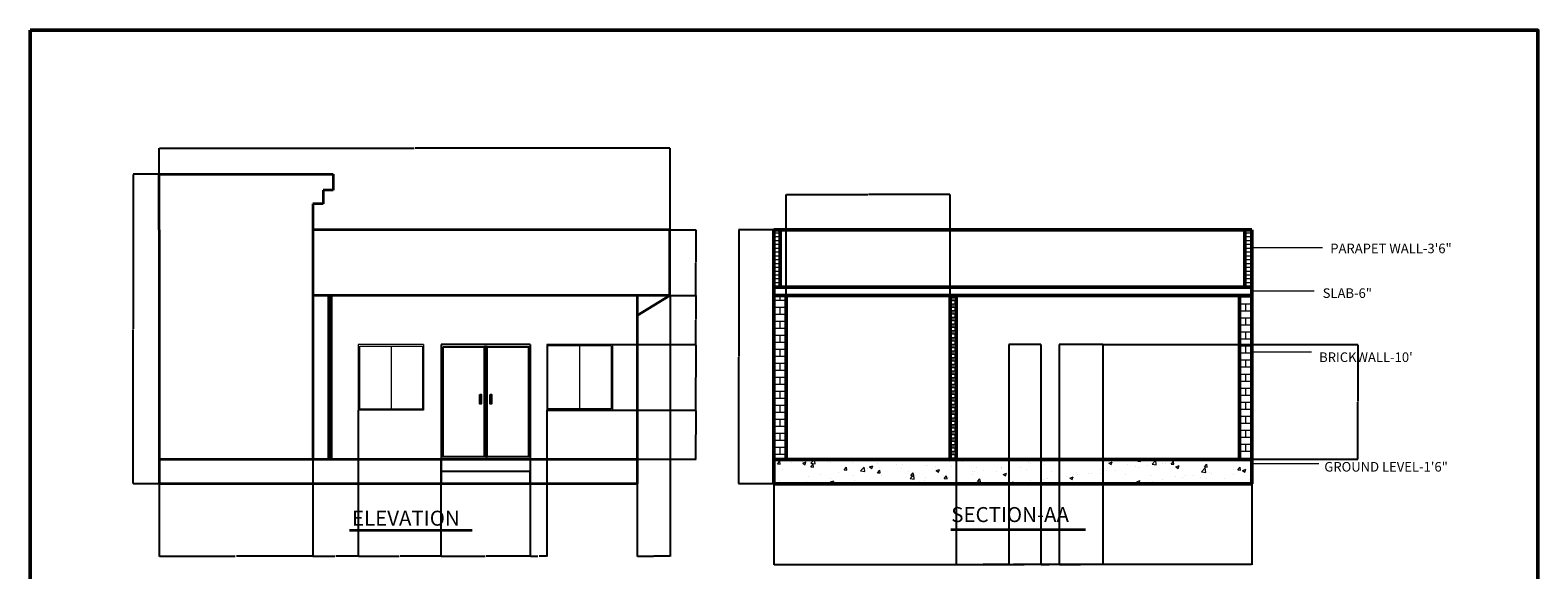
# Model space of a CAD drawing. Units: inches. Extents: x 2268 to 3372, y 1709 to 2892.
# Tile 6 of 6: x 2268 to 3372, y 2497 to 2892. Entities that reach past the tile are written whole.
import ezdxf

# ---------------------------------------------------------------- set-up
doc = ezdxf.new("R2010")
doc.units = ezdxf.units.IN
for name, color, linetype, lineweight in [('A-ANNO-DIMS', 2, 'Continuous', 18), ('A-ANNO-TEXT', 7, 'Continuous', 18), ('A-ANNO-TITL', 7, 'Continuous', 35), ('A-ANNO-TTLB', 7, 'Continuous', 50), ('A-DOOR', 3, 'Continuous', 25), ('A-ELEV', 7, 'Continuous', 35), ('A-FLOR-PATT', 252, 'Continuous', 13), ('A-FLOR-STRS', 7, 'Continuous', 25), ('A-GLAZ', 4, 'Continuous', 18), ('A-SECT', 7, 'Continuous', 50), ('A-WALL-PATT', 252, 'Continuous', 13)]:
    doc.layers.add(name, color=color, linetype=linetype, lineweight=lineweight)
doc.styles.get("Standard").update_dxf_attribs({"font": 'arial.ttf'})
doc.dimstyles.get("Standard").update_dxf_attribs({"dimtxt": 0.18, "dimasz": 0.18, "dimexe": 0.18, "dimexo": 0.0625, "dimgap": 0.09, "dimtad": 0, "dimtih": 1, "dimtoh": 1, "dimdec": 4, "dimzin": 0, "dimdsep": 46, "dimtxsty": 'Standard', "dimcen": 0.09, "dimadec": 0, "dimazin": 0, "dimtfac": 1, "dimtdec": 4, "dimtofl": 0, "dimtmove": 0, "dimatfit": 3, "dimfxl": 1, "dimtolj": 1, "dimtzin": 0, "dimarcsym": 0})

# ---------------------------------------------------------------- blocks, each defined once
blk = doc.blocks.new('*D99')
at = {"layer": 'A-ANNO-DIMS', "color": 0, "lineweight": -2, "transparency": 16777216}
for p, q in [((2362.9, 2786.8), (2362.9, 2806)), ((2363.1, 2805.8), (2549.6, 2805.8)), ((2736.7, 2805.8), (2550.2, 2805.8)), ((2736.9, 2746.2), (2736.9, 2806))]:
    blk.add_line(p, q, dxfattribs=at)
at = {"layer": 'A-ANNO-DIMS', "color": 0, "transparency": 16777216}
for points in [[(2363.1, 2805.9), (2363.1, 2805.8), (2362.9, 2805.8)], [(2736.7, 2805.9), (2736.7, 2805.8), (2736.9, 2805.8)]]:
    blk.add_solid(points, dxfattribs=at)
at = {"layer": 'Defpoints', "color": 0, "transparency": 16777216}
for p in [(2736.9, 2805.8), (2362.9, 2786.8), (2736.9, 2746.2)]:
    blk.add_point(p, dxfattribs=at)
at = {"layer": 'A-ANNO-DIMS', "color": 0, "transparency": 16777216, "insert": (2549.9, 2805.8), "char_height": 0.18, "attachment_point": 5}
blk.add_mtext('\\A1;374', dxfattribs=at)
blk = doc.blocks.new('*D100')
at = {"layer": 'A-ANNO-DIMS', "color": 0, "lineweight": -2, "transparency": 16777216}
for p, q in [((2362.8, 2786.8), (2343.7, 2786.8)), ((2343.8, 2786.6), (2343.8, 2673.7)), ((2343.8, 2560.4), (2343.8, 2673.3)), ((2362.8, 2560.2), (2343.7, 2560.2))]:
    blk.add_line(p, q, dxfattribs=at)
at = {"layer": 'A-ANNO-DIMS', "color": 0, "transparency": 16777216}
for points in [[(2343.8, 2786.6), (2343.9, 2786.6), (2343.8, 2786.8)], [(2343.8, 2560.4), (2343.9, 2560.4), (2343.8, 2560.2)]]:
    blk.add_solid(points, dxfattribs=at)
at = {"layer": 'Defpoints', "color": 0, "transparency": 16777216}
for p in [(2343.8, 2786.8), (2362.9, 2786.8), (2362.9, 2560.2)]:
    blk.add_point(p, dxfattribs=at)
at = {"layer": 'A-ANNO-DIMS', "color": 0, "transparency": 16777216, "insert": (2343.8, 2673.5), "char_height": 0.18, "attachment_point": 5}
blk.add_mtext('\\A1;226.6', dxfattribs=at)
blk = doc.blocks.new('*D101')
at = {"layer": 'A-ANNO-DIMS', "color": 0, "lineweight": -2, "transparency": 16777216}
for p, q in [((2475.3, 2578.1), (2475.3, 2507.1)), ((2362.9, 2560.1), (2362.9, 2507.1)), ((2363.1, 2507.3), (2418.6, 2507.3)), ((2475.1, 2507.3), (2419.5, 2507.3))]:
    blk.add_line(p, q, dxfattribs=at)
at = {"layer": 'A-ANNO-DIMS', "color": 0, "transparency": 16777216}
for points in [[(2363.1, 2507.3), (2363.1, 2507.3), (2362.9, 2507.3)], [(2475.1, 2507.3), (2475.1, 2507.3), (2475.3, 2507.3)]]:
    blk.add_solid(points, dxfattribs=at)
at = {"layer": 'Defpoints', "color": 0, "transparency": 16777216}
for p in [(2475.3, 2578.2), (2362.9, 2560.2), (2475.3, 2507.3)]:
    blk.add_point(p, dxfattribs=at)
at = {"layer": 'A-ANNO-DIMS', "color": 0, "transparency": 16777216, "insert": (2419.1, 2507.3), "char_height": 0.18, "attachment_point": 5}
blk.add_mtext('\\A1;112.37', dxfattribs=at)
blk = doc.blocks.new('*D102')
at = {"layer": 'A-ANNO-DIMS', "color": 0, "lineweight": -2, "transparency": 16777216}
for p, q in [((2508.5, 2614.1), (2508.5, 2507.1)), ((2475.3, 2578.1), (2475.3, 2507.1)), ((2475.4, 2507.3), (2491.5, 2507.3)), ((2508.3, 2507.3), (2492.3, 2507.3))]:
    blk.add_line(p, q, dxfattribs=at)
at = {"layer": 'A-ANNO-DIMS', "color": 0, "transparency": 16777216}
for points in [[(2475.4, 2507.3), (2475.4, 2507.3), (2475.3, 2507.3)], [(2508.3, 2507.3), (2508.3, 2507.3), (2508.5, 2507.3)]]:
    blk.add_solid(points, dxfattribs=at)
at = {"layer": 'Defpoints', "color": 0, "transparency": 16777216}
for p in [(2508.5, 2614.2), (2475.3, 2578.2), (2508.5, 2507.3)]:
    blk.add_point(p, dxfattribs=at)
at = {"layer": 'A-ANNO-DIMS', "color": 0, "transparency": 16777216, "insert": (2491.9, 2507.3), "char_height": 0.18, "attachment_point": 5}
blk.add_mtext('\\A1;33.25', dxfattribs=at)
blk = doc.blocks.new('*D103')
at = {"layer": 'A-ANNO-DIMS', "color": 0, "lineweight": -2, "transparency": 16777216}
for p, q in [((2508.5, 2614.1), (2508.5, 2507.1)), ((2569.2, 2578.1), (2569.2, 2507.1)), ((2508.7, 2507.3), (2538.5, 2507.3)), ((2569.1, 2507.3), (2539.3, 2507.3))]:
    blk.add_line(p, q, dxfattribs=at)
at = {"layer": 'A-ANNO-DIMS', "color": 0, "transparency": 16777216}
for points in [[(2508.7, 2507.3), (2508.7, 2507.3), (2508.5, 2507.3)], [(2569.1, 2507.3), (2569.1, 2507.3), (2569.2, 2507.3)]]:
    blk.add_solid(points, dxfattribs=at)
at = {"layer": 'Defpoints', "color": 0, "transparency": 16777216}
for p in [(2508.5, 2614.2), (2569.2, 2578.2), (2569.2, 2507.3)]:
    blk.add_point(p, dxfattribs=at)
at = {"layer": 'A-ANNO-DIMS', "color": 0, "transparency": 16777216, "insert": (2538.9, 2507.3), "char_height": 0.18, "attachment_point": 5}
blk.add_mtext('\\A1;60.73', dxfattribs=at)
blk = doc.blocks.new('*D104')
at = {"layer": 'A-ANNO-DIMS', "color": 0, "lineweight": -2, "transparency": 16777216}
for p, q in [((2569.2, 2578.1), (2569.2, 2507.1)), ((2634.5, 2578.1), (2634.5, 2507.1)), ((2569.4, 2507.3), (2601.5, 2507.3)), ((2634.4, 2507.3), (2602.3, 2507.3))]:
    blk.add_line(p, q, dxfattribs=at)
at = {"layer": 'A-ANNO-DIMS', "color": 0, "transparency": 16777216}
for points in [[(2569.4, 2507.3), (2569.4, 2507.3), (2569.2, 2507.3)], [(2634.4, 2507.3), (2634.4, 2507.3), (2634.5, 2507.3)]]:
    blk.add_solid(points, dxfattribs=at)
at = {"layer": 'Defpoints', "color": 0, "transparency": 16777216}
for p in [(2569.2, 2578.2), (2634.5, 2578.2), (2634.5, 2507.3)]:
    blk.add_point(p, dxfattribs=at)
at = {"layer": 'A-ANNO-DIMS', "color": 0, "transparency": 16777216, "insert": (2601.9, 2507.3), "char_height": 0.18, "attachment_point": 5}
blk.add_mtext('\\A1;65.29', dxfattribs=at)
blk = doc.blocks.new('*D105')
at = {"layer": 'A-ANNO-DIMS', "color": 0, "lineweight": -2, "transparency": 16777216}
for p, q in [((2646.7, 2614.1), (2646.7, 2507.1)), ((2634.5, 2578.1), (2634.5, 2507.1)), ((2634.7, 2507.3), (2640.2, 2507.3)), ((2646.5, 2507.3), (2641.1, 2507.3))]:
    blk.add_line(p, q, dxfattribs=at)
at = {"layer": 'A-ANNO-DIMS', "color": 0, "transparency": 16777216}
for points in [[(2634.7, 2507.3), (2634.7, 2507.3), (2634.5, 2507.3)], [(2646.5, 2507.3), (2646.5, 2507.3), (2646.7, 2507.3)]]:
    blk.add_solid(points, dxfattribs=at)
at = {"layer": 'Defpoints', "color": 0, "transparency": 16777216}
for p in [(2646.7, 2614.2), (2634.5, 2578.2), (2646.7, 2507.3)]:
    blk.add_point(p, dxfattribs=at)
at = {"layer": 'A-ANNO-DIMS', "color": 0, "transparency": 16777216, "insert": (2640.6, 2507.3), "char_height": 0.18, "attachment_point": 5}
blk.add_mtext('\\A1;12.153', dxfattribs=at)
blk = doc.blocks.new('*D106')
at = {"layer": 'A-ANNO-DIMS', "color": 0, "lineweight": -2, "transparency": 16777216}
for p, q in [((2736.9, 2698.1), (2736.9, 2507.1)), ((2712.9, 2560.1), (2712.9, 2507.1)), ((2713.1, 2507.3), (2724.7, 2507.3)), ((2736.7, 2507.3), (2725.1, 2507.3))]:
    blk.add_line(p, q, dxfattribs=at)
at = {"layer": 'A-ANNO-DIMS', "color": 0, "transparency": 16777216}
for points in [[(2713.1, 2507.3), (2713.1, 2507.3), (2712.9, 2507.3)], [(2736.7, 2507.3), (2736.7, 2507.3), (2736.9, 2507.3)]]:
    blk.add_solid(points, dxfattribs=at)
at = {"layer": 'Defpoints', "color": 0, "transparency": 16777216}
for p in [(2736.9, 2698.2), (2712.9, 2560.2), (2736.9, 2507.3)]:
    blk.add_point(p, dxfattribs=at)
at = {"layer": 'A-ANNO-DIMS', "color": 0, "transparency": 16777216, "insert": (2724.9, 2507.3), "char_height": 0.18, "attachment_point": 5}
blk.add_mtext('\\A1;24', dxfattribs=at)
blk = doc.blocks.new('*D107')
at = {"layer": 'A-ANNO-DIMS', "color": 0, "lineweight": -2, "transparency": 16777216}
for p, q in [((2694.7, 2662.2), (2756.1, 2662.2)), ((2755.9, 2662), (2755.9, 2638.4)), ((2755.9, 2614.4), (2755.9, 2638)), ((2646.7, 2614.2), (2756.1, 2614.2))]:
    blk.add_line(p, q, dxfattribs=at)
at = {"layer": 'A-ANNO-DIMS', "color": 0, "transparency": 16777216}
for points in [[(2755.9, 2662), (2756, 2662), (2755.9, 2662.2)], [(2755.9, 2614.4), (2756, 2614.4), (2755.9, 2614.2)]]:
    blk.add_solid(points, dxfattribs=at)
at = {"layer": 'Defpoints', "color": 0, "transparency": 16777216}
for p in [(2694.7, 2662.2), (2755.9, 2662.2), (2646.7, 2614.2)]:
    blk.add_point(p, dxfattribs=at)
at = {"layer": 'A-ANNO-DIMS', "color": 0, "transparency": 16777216, "insert": (2755.9, 2638.2), "char_height": 0.18, "attachment_point": 5}
blk.add_mtext('\\A1;48', dxfattribs=at)
blk = doc.blocks.new('*D108')
at = {"layer": 'A-ANNO-DIMS', "color": 0, "lineweight": -2, "transparency": 16777216}
for p, q in [((2694.7, 2614.2), (2756.1, 2614.2)), ((2755.9, 2614), (2755.9, 2596.4)), ((2755.9, 2578.4), (2755.9, 2596)), ((2713, 2578.2), (2756.1, 2578.2))]:
    blk.add_line(p, q, dxfattribs=at)
at = {"layer": 'A-ANNO-DIMS', "color": 0, "transparency": 16777216}
for points in [[(2755.9, 2614), (2756, 2614), (2755.9, 2614.2)], [(2755.9, 2578.4), (2756, 2578.4), (2755.9, 2578.2)]]:
    blk.add_solid(points, dxfattribs=at)
at = {"layer": 'Defpoints', "color": 0, "transparency": 16777216}
for p in [(2694.7, 2614.2), (2755.9, 2614.2), (2712.9, 2578.2)]:
    blk.add_point(p, dxfattribs=at)
at = {"layer": 'A-ANNO-DIMS', "color": 0, "transparency": 16777216, "insert": (2755.9, 2596.2), "char_height": 0.18, "attachment_point": 5}
blk.add_mtext('\\A1;36', dxfattribs=at)
blk = doc.blocks.new('*D109')
at = {"layer": 'A-ANNO-DIMS', "color": 0, "lineweight": -2, "transparency": 16777216}
for p, q in [((2737, 2698.2), (2756.1, 2698.2)), ((2755.9, 2698), (2755.9, 2680.4)), ((2755.9, 2662.4), (2755.9, 2680)), ((2694.7, 2662.2), (2756.1, 2662.2))]:
    blk.add_line(p, q, dxfattribs=at)
at = {"layer": 'A-ANNO-DIMS', "color": 0, "transparency": 16777216}
for points in [[(2755.9, 2698), (2756, 2698), (2755.9, 2698.2)], [(2755.9, 2662.4), (2756, 2662.4), (2755.9, 2662.2)]]:
    blk.add_solid(points, dxfattribs=at)
at = {"layer": 'Defpoints', "color": 0, "transparency": 16777216}
for p in [(2736.9, 2698.2), (2755.9, 2698.2), (2694.7, 2662.2)]:
    blk.add_point(p, dxfattribs=at)
at = {"layer": 'A-ANNO-DIMS', "color": 0, "transparency": 16777216, "insert": (2755.9, 2680.2), "char_height": 0.18, "attachment_point": 5}
blk.add_mtext('\\A1;36', dxfattribs=at)
blk = doc.blocks.new('*D110')
at = {"layer": 'A-ANNO-DIMS', "color": 0, "lineweight": -2, "transparency": 16777216}
for p, q in [((2737, 2746.2), (2756.1, 2746.2)), ((2755.9, 2746), (2755.9, 2722.4)), ((2755.9, 2698.4), (2755.9, 2722)), ((2737, 2698.2), (2756.1, 2698.2))]:
    blk.add_line(p, q, dxfattribs=at)
at = {"layer": 'A-ANNO-DIMS', "color": 0, "transparency": 16777216}
for points in [[(2755.9, 2746), (2756, 2746), (2755.9, 2746.2)], [(2755.9, 2698.4), (2756, 2698.4), (2755.9, 2698.2)]]:
    blk.add_solid(points, dxfattribs=at)
at = {"layer": 'Defpoints', "color": 0, "transparency": 16777216}
for p in [(2736.9, 2746.2), (2755.9, 2746.2), (2736.9, 2698.2)]:
    blk.add_point(p, dxfattribs=at)
at = {"layer": 'A-ANNO-DIMS', "color": 0, "transparency": 16777216, "insert": (2755.9, 2722.2), "char_height": 0.18, "attachment_point": 5}
blk.add_mtext('\\A1;48', dxfattribs=at)
blk = doc.blocks.new('*D111')
at = {"layer": 'A-ANNO-DIMS', "color": 0, "lineweight": -2, "transparency": 16777216}
for p, q in [((2813, 2560.1), (2813, 2501)), ((3163, 2560.1), (3163, 2501)), ((2813.2, 2501.2), (2987.7, 2501.2)), ((3162.8, 2501.2), (2988.3, 2501.2))]:
    blk.add_line(p, q, dxfattribs=at)
at = {"layer": 'A-ANNO-DIMS', "color": 0, "transparency": 16777216}
for points in [[(2813.2, 2501.3), (2813.2, 2501.2), (2813, 2501.2)], [(3162.8, 2501.3), (3162.8, 2501.2), (3163, 2501.2)]]:
    blk.add_solid(points, dxfattribs=at)
at = {"layer": 'Defpoints', "color": 0, "transparency": 16777216}
for p in [(2813, 2560.2), (3163, 2560.2), (3163, 2501.2)]:
    blk.add_point(p, dxfattribs=at)
at = {"layer": 'A-ANNO-DIMS', "color": 0, "transparency": 16777216, "insert": (2988, 2501.2), "char_height": 0.18, "attachment_point": 5}
blk.add_mtext('\\A1;350', dxfattribs=at)
blk = doc.blocks.new('*D112')
at = {"layer": 'A-ANNO-DIMS', "color": 0, "lineweight": -2, "transparency": 16777216}
for p, q in [((2812.9, 2746.2), (2787.1, 2746.2)), ((2787.3, 2746), (2787.3, 2653.4)), ((2787.3, 2560.4), (2787.3, 2653)), ((2812.9, 2560.2), (2787.1, 2560.2))]:
    blk.add_line(p, q, dxfattribs=at)
at = {"layer": 'A-ANNO-DIMS', "color": 0, "transparency": 16777216}
for points in [[(2787.3, 2746), (2787.3, 2746), (2787.3, 2746.2)], [(2787.3, 2560.4), (2787.3, 2560.4), (2787.3, 2560.2)]]:
    blk.add_solid(points, dxfattribs=at)
at = {"layer": 'Defpoints', "color": 0, "transparency": 16777216}
for p in [(2787.3, 2746.2), (2813, 2746.2), (2813, 2560.2)]:
    blk.add_point(p, dxfattribs=at)
at = {"layer": 'A-ANNO-DIMS', "color": 0, "transparency": 16777216, "insert": (2787.3, 2653.2), "char_height": 0.18, "attachment_point": 5}
blk.add_mtext('\\A1;186', dxfattribs=at)
blk = doc.blocks.new('*D113')
at = {"layer": 'A-ANNO-DIMS', "color": 0, "lineweight": -2, "transparency": 16777216}
for p, q in [((2822, 2698.2), (2822, 2772.1)), ((2822.2, 2771.9), (2881.7, 2771.9)), ((2941.8, 2771.9), (2882.3, 2771.9)), ((2942, 2698.2), (2942, 2772.1))]:
    blk.add_line(p, q, dxfattribs=at)
at = {"layer": 'A-ANNO-DIMS', "color": 0, "transparency": 16777216}
for points in [[(2822.2, 2771.9), (2822.2, 2771.9), (2822, 2771.9)], [(2941.8, 2771.9), (2941.8, 2771.9), (2942, 2771.9)]]:
    blk.add_solid(points, dxfattribs=at)
at = {"layer": 'Defpoints', "color": 0, "transparency": 16777216}
for p in [(2942, 2771.9), (2822, 2698.2), (2942, 2698.2)]:
    blk.add_point(p, dxfattribs=at)
at = {"layer": 'A-ANNO-DIMS', "color": 0, "transparency": 16777216, "insert": (2882, 2771.9), "char_height": 0.18, "attachment_point": 5}
blk.add_mtext('\\A1;120', dxfattribs=at)
blk = doc.blocks.new('*D114')
at = {"layer": 'A-ANNO-DIMS', "color": 0, "lineweight": -2, "transparency": 16777216}
for p, q in [((2946.5, 2578.1), (2946.5, 2501)), ((2985, 2578.1), (2985, 2501)), ((2946.7, 2501.2), (2965.3, 2501.2)), ((2984.8, 2501.2), (2966.2, 2501.2))]:
    blk.add_line(p, q, dxfattribs=at)
at = {"layer": 'A-ANNO-DIMS', "color": 0, "transparency": 16777216}
for points in [[(2946.7, 2501.3), (2946.7, 2501.2), (2946.5, 2501.2)], [(2984.8, 2501.3), (2984.8, 2501.2), (2985, 2501.2)]]:
    blk.add_solid(points, dxfattribs=at)
at = {"layer": 'Defpoints', "color": 0, "transparency": 16777216}
for p in [(2946.5, 2578.2), (2985, 2578.2), (2985, 2501.2)]:
    blk.add_point(p, dxfattribs=at)
at = {"layer": 'A-ANNO-DIMS', "color": 0, "transparency": 16777216, "insert": (2965.7, 2501.2), "char_height": 0.18, "attachment_point": 5}
blk.add_mtext('\\A1;38.486', dxfattribs=at)
blk = doc.blocks.new('*D115')
at = {"layer": 'A-ANNO-DIMS', "color": 0, "lineweight": -2, "transparency": 16777216}
for p, q in [((2985, 2578.1), (2985, 2501)), ((3008.4, 2578.1), (3008.4, 2501)), ((2985.2, 2501.2), (2996.2, 2501.2)), ((3008.2, 2501.2), (2997.2, 2501.2))]:
    blk.add_line(p, q, dxfattribs=at)
at = {"layer": 'A-ANNO-DIMS', "color": 0, "transparency": 16777216}
for points in [[(2985.2, 2501.3), (2985.2, 2501.2), (2985, 2501.2)], [(3008.2, 2501.3), (3008.2, 2501.2), (3008.4, 2501.2)]]:
    blk.add_solid(points, dxfattribs=at)
at = {"layer": 'Defpoints', "color": 0, "transparency": 16777216}
for p in [(2985, 2578.2), (3008.4, 2578.2), (3008.4, 2501.2)]:
    blk.add_point(p, dxfattribs=at)
at = {"layer": 'A-ANNO-DIMS', "color": 0, "transparency": 16777216, "insert": (2996.7, 2501.2), "char_height": 0.18, "attachment_point": 5}
blk.add_mtext('\\A1;23.404', dxfattribs=at)
blk = doc.blocks.new('*D116')
at = {"layer": 'A-ANNO-DIMS', "color": 0, "lineweight": -2, "transparency": 16777216}
for p, q in [((3008.4, 2578.1), (3008.4, 2501)), ((3021.8, 2578.1), (3021.8, 2501)), ((3008.6, 2501.2), (3014.6, 2501.2)), ((3021.6, 2501.2), (3015.5, 2501.2))]:
    blk.add_line(p, q, dxfattribs=at)
at = {"layer": 'A-ANNO-DIMS', "color": 0, "transparency": 16777216}
for points in [[(3008.6, 2501.3), (3008.6, 2501.2), (3008.4, 2501.2)], [(3021.6, 2501.3), (3021.6, 2501.2), (3021.8, 2501.2)]]:
    blk.add_solid(points, dxfattribs=at)
at = {"layer": 'Defpoints', "color": 0, "transparency": 16777216}
for p in [(3008.4, 2578.2), (3021.8, 2578.2), (3021.8, 2501.2)]:
    blk.add_point(p, dxfattribs=at)
at = {"layer": 'A-ANNO-DIMS', "color": 0, "transparency": 16777216, "insert": (3015.1, 2501.2), "char_height": 0.18, "attachment_point": 5}
blk.add_mtext('\\A1;13.395', dxfattribs=at)
blk = doc.blocks.new('*D117')
at = {"layer": 'A-ANNO-DIMS', "color": 0, "lineweight": -2, "transparency": 16777216}
for p, q in [((3021.8, 2578.1), (3021.8, 2501)), ((3053.9, 2578.1), (3053.9, 2501)), ((3022, 2501.2), (3037.5, 2501.2)), ((3053.7, 2501.2), (3038.2, 2501.2))]:
    blk.add_line(p, q, dxfattribs=at)
at = {"layer": 'A-ANNO-DIMS', "color": 0, "transparency": 16777216}
for points in [[(3022, 2501.3), (3022, 2501.2), (3021.8, 2501.2)], [(3053.7, 2501.3), (3053.7, 2501.2), (3053.9, 2501.2)]]:
    blk.add_solid(points, dxfattribs=at)
at = {"layer": 'Defpoints', "color": 0, "transparency": 16777216}
for p in [(3021.8, 2578.2), (3053.9, 2578.2), (3053.9, 2501.2)]:
    blk.add_point(p, dxfattribs=at)
at = {"layer": 'A-ANNO-DIMS', "color": 0, "transparency": 16777216, "insert": (3037.9, 2501.2), "char_height": 0.18, "attachment_point": 5}
blk.add_mtext('\\A1;32.14', dxfattribs=at)
blk = doc.blocks.new('*D118')
at = {"layer": 'A-ANNO-DIMS', "color": 0, "lineweight": -2, "transparency": 16777216}
for p, q in [((3054, 2662.2), (3240.6, 2662.2)), ((3240.5, 2662), (3240.5, 2620.4)), ((3240.5, 2578.4), (3240.5, 2620)), ((3054, 2578.2), (3240.6, 2578.2))]:
    blk.add_line(p, q, dxfattribs=at)
at = {"layer": 'A-ANNO-DIMS', "color": 0, "transparency": 16777216}
for points in [[(3240.4, 2662), (3240.5, 2662), (3240.5, 2662.2)], [(3240.4, 2578.4), (3240.5, 2578.4), (3240.5, 2578.2)]]:
    blk.add_solid(points, dxfattribs=at)
at = {"layer": 'Defpoints', "color": 0, "transparency": 16777216}
for p in [(3053.9, 2662.2), (3240.5, 2662.2), (3053.9, 2578.2)]:
    blk.add_point(p, dxfattribs=at)
at = {"layer": 'A-ANNO-DIMS', "color": 0, "transparency": 16777216, "insert": (3240.5, 2620.2), "char_height": 0.18, "attachment_point": 5}
blk.add_mtext('\\A1;84', dxfattribs=at)

msp = doc.modelspace()

# ---------------------------------------------------------------- hatches: boundary and pattern name
at = {"layer": 'A-FLOR-PATT'}
h = msp.add_hatch(dxfattribs=at)
h.set_pattern_fill('AR-CONC', color=256, scale=0.134, style=0)
h.paths.add_polyline_path([(2813.001, 2560.1868), (3163.001, 2560.1868), (3163.001, 2578.1868), (2813.001, 2578.1868)])
at = {"layer": 'A-WALL-PATT'}
h = msp.add_hatch(dxfattribs=at)
h.set_pattern_fill('LINE', color=256, scale=0.88189, style=0)
h.paths.add_polyline_path([(2813.001, 2704.1868), (2817.6812, 2704.1868), (2817.6812, 2746.1868), (2813.001, 2746.1868)])
h = msp.add_hatch(dxfattribs=at)
h.set_pattern_fill('LINE', color=256, scale=0.88189, style=0)
h.paths.add_polyline_path([(3157.7911, 2704.1868), (3163.001, 2704.1868), (3163.001, 2746.1868), (3157.7911, 2746.1868)])
h = msp.add_hatch(dxfattribs=at)
h.set_pattern_fill('BRICK', color=256, scale=0.80673, style=0)
h.paths.add_polyline_path([(2813.001, 2578.1868), (2822.001, 2578.1868), (2822.001, 2698.1868), (2813.001, 2698.1868)])
h = msp.add_hatch(dxfattribs=at)
h.set_pattern_fill('BRICK', color=256, scale=0.3857417, style=0)
h.paths.add_polyline_path([(2942.001, 2578.1868), (2946.501, 2578.1868), (2946.501, 2698.1868), (2942.001, 2698.1868)])
h = msp.add_hatch(dxfattribs=at)
h.set_pattern_fill('BRICK', color=256, scale=0.80747, style=0)
h.paths.add_polyline_path([(3154.001, 2578.1868), (3163.001, 2578.1868), (3163.001, 2698.1868), (3154.001, 2698.1868)])

# ---------------------------------------------------------------- linework, layer by layer
at = {"layer": 'A-ANNO-TEXT'}
for p, q in [((3163.001, 2733.2345), (3214.7573, 2733.2345)), ((3163.001, 2701.4852), (3208.4818, 2701.4852)), ((3163.001, 2656.8404), (3206.5729, 2656.8404)), ((3163.001, 2575.0552), (3212.0318, 2575.0552))]:
    msp.add_line(p, q, dxfattribs=at)
at = {"layer": 'A-ANNO-TITL'}
for p, q in [((2502.209, 2526.3436), (2592.0256, 2526.3436)), ((2942.4583, 2526.9258), (3041.1812, 2526.9258))]:
    msp.add_line(p, q, dxfattribs=at)
at = {"layer": 'A-ANNO-TTLB'}
msp.add_lwpolyline([(2268.3884, 2892.2471), (3372.3464, 2892.2471), (3372.3464, 1709.0755), (2268.3884, 1709.0755)], close=True, dxfattribs=at)
at = {"layer": 'A-DOOR'}
for p, q in [((2569.2467, 2662.1868), (2569.2467, 2578.1868)), ((2634.5318, 2662.1868), (2569.2467, 2662.1868)), ((2601.9304, 2660.6318), (2600.9304, 2660.6318)), ((2600.9304, 2660.6318), (2600.9304, 2579.9595)), ((2601.9304, 2660.6318), (2601.9304, 2579.9595)), ((2602.9304, 2660.6318), (2601.9304, 2660.6318)), ((2602.9304, 2579.9595), (2602.9304, 2660.6318)), ((2634.5318, 2662.1868), (2634.5318, 2578.1868)), ((2984.9866, 2662.1868), (2984.9866, 2578.1868)), ((3008.3904, 2662.1868), (2984.9866, 2662.1868)), ((3008.3904, 2662.1868), (3008.3904, 2578.1868)), ((3021.7859, 2662.1868), (3021.7859, 2578.1868)), ((3053.9275, 2662.1868), (3021.7859, 2662.1868)), ((3053.9275, 2662.1868), (3053.9275, 2578.1868)), ((2601.9304, 2579.9595), (2602.9304, 2579.9595))]:
    msp.add_line(p, q, dxfattribs=at)
for points in [[(2570.6907, 2660.6318), (2633.1702, 2660.6318), (2633.1702, 2579.9595), (2570.6907, 2579.9595)], [(2597.5773, 2625.6994), (2598.6814, 2625.6994), (2598.6814, 2618.7197), (2597.5773, 2618.7197)], [(2605.167, 2625.6994), (2606.2712, 2625.6994), (2606.2712, 2618.7197), (2605.167, 2618.7197)], [(2605.167, 2625.6994), (2606.2712, 2625.6994), (2606.2712, 2618.7197), (2605.167, 2618.7197)]]:
    msp.add_lwpolyline(points, close=True, dxfattribs=at)
at = {"layer": 'A-ELEV'}
for p, q in [((2362.8943, 2746.1868), (2362.8943, 2786.782)), ((2362.8943, 2786.782), (2490.3619, 2786.782)), ((2490.3619, 2786.782), (2490.3619, 2775.2614)), ((2490.3619, 2775.2614), (2482.9423, 2775.2614)), ((2482.9423, 2775.2614), (2482.9423, 2765.097)), ((2482.9423, 2765.097), (2475.2688, 2765.097)), ((2475.2688, 2765.097), (2475.2688, 2746.1868)), ((2362.8943, 2746.1868), (2362.8943, 2560.1868)), ((2736.8943, 2746.1868), (2475.2688, 2746.1868)), ((2475.2688, 2746.1868), (2475.2688, 2578.1868)), ((2736.8943, 2698.1868), (2736.8943, 2746.1868)), ((2488.9571, 2698.1868), (2475.2688, 2698.1868)), ((2488.9571, 2698.1868), (2486.9571, 2698.1868)), ((2486.9571, 2698.1868), (2486.9571, 2578.1868)), ((2736.8943, 2698.1868), (2488.9571, 2698.1868)), ((2488.9571, 2578.1868), (2488.9571, 2698.1868)), ((2712.8943, 2698.1868), (2712.8943, 2560.1868)), ((2736.8943, 2698.1868), (2712.8943, 2683.3831)), ((2712.8943, 2578.1868), (2362.8943, 2578.1868)), ((2712.8943, 2560.1868), (2362.8943, 2560.1868))]:
    msp.add_line(p, q, dxfattribs=at)
at = {"layer": 'A-FLOR-STRS'}
for p, q in [((2569.2467, 2578.1868), (2569.2467, 2560.1868)), ((2634.5318, 2578.1868), (2634.5318, 2560.1868)), ((2634.5318, 2569.1868), (2569.2467, 2569.1868)), ((2634.5318, 2560.1868), (2634.5318, 2569.1868))]:
    msp.add_line(p, q, dxfattribs=at)
at = {"layer": 'A-GLAZ'}
for p, q in [((2508.5215, 2662.1868), (2508.5215, 2614.1868)), ((2556.5215, 2662.1868), (2508.5215, 2662.1868)), ((2532.7598, 2661.0404), (2532.7598, 2614.9718)), ((2556.5215, 2662.1868), (2556.5215, 2614.1868)), ((2646.6845, 2662.1868), (2646.6845, 2614.1868)), ((2694.6845, 2662.1868), (2646.6845, 2662.1868)), ((2670.6544, 2661.411), (2670.6544, 2615.2501)), ((2694.6845, 2662.1868), (2694.6845, 2614.1868)), ((2556.5215, 2614.1868), (2508.5215, 2614.1868)), ((2694.6845, 2614.1868), (2646.6845, 2614.1868))]:
    msp.add_line(p, q, dxfattribs=at)
for points in [[(2509.7776, 2661.0404), (2555.742, 2661.0404), (2555.742, 2614.9718), (2509.7776, 2614.9718)], [(2647.4927, 2661.411), (2693.8162, 2661.411), (2693.8162, 2615.2501), (2647.4927, 2615.2501)]]:
    msp.add_lwpolyline(points, close=True, dxfattribs=at)
at = {"layer": 'A-SECT'}
for p, q in [((2813.001, 2746.1868), (2813.001, 2560.1868)), ((3163.001, 2746.1868), (2813.001, 2746.1868)), ((2817.6812, 2704.1868), (2817.6812, 2746.1868)), ((3157.7911, 2704.1868), (3157.7911, 2746.1868)), ((3163.001, 2746.1868), (3163.001, 2560.1868)), ((3163.001, 2704.1868), (2813.001, 2704.1868)), ((3163.001, 2698.1868), (2813.001, 2698.1868)), ((2822.001, 2698.1868), (2822.001, 2578.1868)), ((2942.001, 2698.1868), (2942.001, 2578.1868)), ((2946.501, 2698.1868), (2946.501, 2578.1868)), ((3154.001, 2698.1868), (3154.001, 2578.1868)), ((3163.001, 2578.1868), (2813.001, 2578.1868)), ((3163.001, 2560.1868), (2813.001, 2560.1868))]:
    msp.add_line(p, q, dxfattribs=at)

# ---------------------------------------------------------------- texts
at = {"layer": 'A-ANNO-TEXT', "char_height": 7, "attachment_point": 1}
for s, width, insert in [('PARAPET WALL-3\'6"', 228.095751, (3220.3641, 2736.0218)), ('SLAB-6"', 73.386831, (3214.8036, 2703.2982)), ("BRICKWALL-10'", 72.583254, (3212.1972, 2656.439)), ('GROUND LEVEL-1\'6"', 104.232109, (3216.0152, 2576.242))]:
    msp.add_mtext_dynamic_manual_height_columns(s, width=width, gutter_width=12.5, heights=[0], dxfattribs=dict(at, insert=insert))
at = {"layer": 'A-ANNO-TITL', "char_height": 11, "attachment_point": 1}
for s, width, insert in [('ELEVATION', 248.660819, (2504.0082, 2540.6159)), ('SECTION-AA', 156.391349, (2942.8373, 2543.2613))]:
    msp.add_mtext_dynamic_manual_height_columns(s, width=width, gutter_width=12.5, heights=[0], dxfattribs=dict(at, insert=insert))

# ---------------------------------------------------------------- dimensions: what is measured, and where the dimension line sits
at = {"layer": 'A-ANNO-DIMS'}
for base, p1, p2, override, picture, middle in [((2736.8943, 2805.832), (2362.8943, 2786.782), (2736.8943, 2746.1868), {"dimdec": 0, "dimlfac": 1, "dimrnd": 0, "dimzin": 0, "dimdsep": 46, "dimlunit": 2}, '*D99', (2549.8943, 2805.832)), ((2942.001, 2771.8868), (2822.001, 2698.1868), (2942.001, 2698.1868), {"dimdec": 0, "dimlfac": 1, "dimrnd": 0, "dimzin": 0, "dimdsep": 46, "dimlunit": 2}, '*D113', (2882.001, 2771.8868)), ((2736.8943, 2507.2936), (2712.8943, 2560.1868), (2736.8943, 2698.1868), {"dimdec": 0, "dimlfac": 1, "dimrnd": 0, "dimzin": 0, "dimdsep": 46, "dimlunit": 2}, '*D106', (2724.8943, 2507.2936)), ((2508.5215, 2507.2936), (2475.2688, 2578.1868), (2508.5215, 2614.1868), {"dimdec": 2, "dimlfac": 1, "dimrnd": 0, "dimzin": 0, "dimdsep": 46, "dimlunit": 2}, '*D102', (2491.8952, 2507.2936)), ((2569.2467, 2507.2936), (2508.5215, 2614.1868), (2569.2467, 2578.1868), {"dimdec": 2, "dimlfac": 1, "dimrnd": 0, "dimzin": 0, "dimdsep": 46, "dimlunit": 2}, '*D103', (2538.8841, 2507.2936)), ((2646.6845, 2507.2936), (2634.5318, 2578.1868), (2646.6845, 2614.1868), {"dimdec": 3, "dimlfac": 1, "dimrnd": 0, "dimzin": 0, "dimdsep": 46, "dimlunit": 2}, '*D105', (2640.6082, 2507.2936)), ((2475.2688, 2507.2936), (2362.8943, 2560.1868), (2475.2688, 2578.1868), {"dimdec": 2, "dimlfac": 1, "dimrnd": 0, "dimzin": 0, "dimdsep": 46, "dimlunit": 2}, '*D101', (2419.0815, 2507.2936)), ((2634.5318, 2507.2936), (2569.2467, 2578.1868), (2634.5318, 2578.1868), {"dimdec": 2, "dimlfac": 1, "dimrnd": 0, "dimzin": 0, "dimdsep": 46, "dimlunit": 2}, '*D104', (2601.8893, 2507.2936)), ((2984.9866, 2501.2258), (2946.501, 2578.1868), (2984.9866, 2578.1868), {"dimdec": 3, "dimlfac": 1, "dimrnd": 0, "dimzin": 0, "dimdsep": 46, "dimlunit": 2}, '*D114', (2965.7438, 2501.2258)), ((3008.3904, 2501.2258), (2984.9866, 2578.1868), (3008.3904, 2578.1868), {"dimdec": 3, "dimlfac": 1, "dimrnd": 0, "dimzin": 0, "dimdsep": 46, "dimlunit": 2}, '*D115', (2996.6885, 2501.2258)), ((3021.78586, 2501.22583), (3008.39037, 2578.18679), (3021.78586, 2578.18679), {"dimdec": 3, "dimlfac": 1, "dimrnd": 0, "dimzin": 0, "dimdsep": 46, "dimlunit": 2}, '*D116', (3015.08812, 2501.22583)), ((3053.9275, 2501.2258), (3021.7859, 2578.1868), (3053.9275, 2578.1868), {"dimdec": 2, "dimlfac": 1, "dimrnd": 0, "dimzin": 0, "dimdsep": 46, "dimlunit": 2}, '*D117', (3037.8567, 2501.2258)), ((3163.001, 2501.2258), (2813.001, 2560.1868), (3163.001, 2560.1868), {"dimdec": 0, "dimlfac": 1, "dimrnd": 0, "dimzin": 0, "dimdsep": 46, "dimlunit": 2}, '*D111', (2988.001, 2501.2258))]:
    dim = msp.add_linear_dim(base=base, p1=p1, p2=p2, dimstyle='Standard', override=override, dxfattribs=at)
    dim.commit()
    dim.dimension.update_dxf_attribs({"geometry": picture, "text_midpoint": middle})
for base, p1, p2, override, picture, middle in [((2343.8443, 2786.782), (2362.8943, 2560.1868), (2362.8943, 2786.782), {"dimdec": 1, "dimlfac": 1, "dimrnd": 0, "dimzin": 0, "dimdsep": 46, "dimlunit": 2}, '*D100', (2343.8443, 2673.4844)), ((2755.9443, 2746.1868), (2736.8943, 2698.1868), (2736.8943, 2746.1868), {"dimdec": 0, "dimlfac": 1, "dimrnd": 0, "dimzin": 0, "dimdsep": 46, "dimlunit": 2}, '*D110', (2755.9443, 2722.1868)), ((2787.301, 2746.1868), (2813.001, 2560.1868), (2813.001, 2746.1868), {"dimdec": 0, "dimlfac": 1, "dimrnd": 0, "dimzin": 0, "dimdsep": 46, "dimlunit": 2}, '*D112', (2787.301, 2653.1868)), ((2755.9443, 2698.1868), (2694.6845, 2662.1868), (2736.8943, 2698.1868), {"dimdec": 0, "dimlfac": 1, "dimrnd": 0, "dimzin": 0, "dimdsep": 46, "dimlunit": 2}, '*D109', (2755.9443, 2680.1868)), ((2755.9443, 2662.1868), (2646.6845, 2614.1868), (2694.6845, 2662.1868), {"dimdec": 0, "dimlfac": 1, "dimrnd": 0, "dimzin": 0, "dimdsep": 46, "dimlunit": 2}, '*D107', (2755.9443, 2638.1868)), ((3240.4573, 2662.1868), (3053.9275, 2578.1868), (3053.9275, 2662.1868), {"dimdec": 0, "dimlfac": 1, "dimrnd": 0, "dimzin": 0, "dimdsep": 46, "dimlunit": 2}, '*D118', (3240.4573, 2620.1868)), ((2755.9443, 2614.1868), (2712.8943, 2578.1868), (2694.6845, 2614.1868), {"dimdec": 0, "dimlfac": 1, "dimrnd": 0, "dimzin": 0, "dimdsep": 46, "dimlunit": 2}, '*D108', (2755.9443, 2596.1868))]:
    dim = msp.add_linear_dim(base=base, p1=p1, p2=p2, angle=90, dimstyle='Standard', override=override, dxfattribs=at)
    dim.commit()
    dim.dimension.update_dxf_attribs({"geometry": picture, "text_midpoint": middle})

doc.saveas('drawing.dxf')
